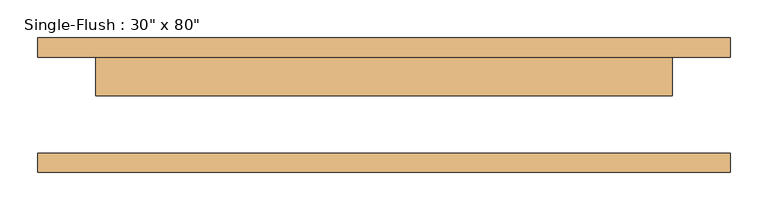
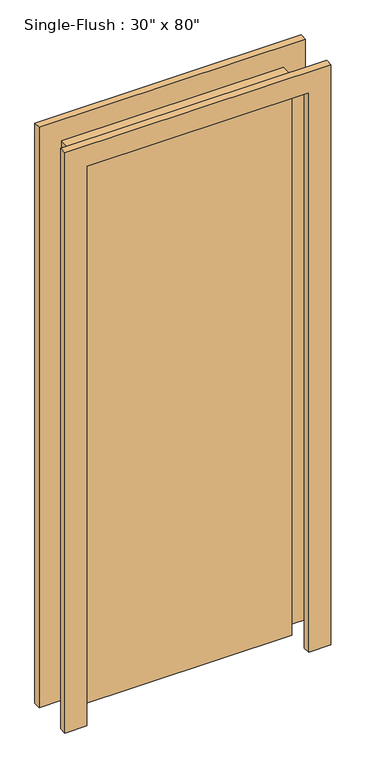
"""IFC4 building model written with IfcOpenShell, lengths in millimetres: door geometry."""

from ifc_helpers import new_model, si_unit, frame, origin, origin_with_axes, place, context, project, spatial, polyline, outline, extrude, source, transform, mapped, element, save


def door_1fe7f57d(model_context):
    return source(origin(), model_context, "Body", "SweptSolid", [
        extrude(outline(polyline([(2108.2, -457.2), (0.0, -457.2), (0.0, -381.0), (2032.0, -381.0), (2032.0, 381.0), (0.0, 381.0), (0.0, 457.2), (2108.2, 457.2), (2108.2, -457.2)])), frame((0.0, 63.5, 0.0), z_axis=(0.0, 1.0, 0.0), x_axis=(0.0, 0.0, 1.0)), (0.0, 0.0, 1.0), 25.4),
        extrude(outline(polyline([(2108.2, 457.2), (2108.2, -457.2), (0.0, -457.2), (0.0, -381.0), (2032.0, -381.0), (2032.0, 381.0), (0.0, 381.0), (0.0, 457.2), (2108.2, 457.2)])), frame((0.0, -88.9, 0.0), z_axis=(0.0, 1.0, 0.0), x_axis=(0.0, 0.0, 1.0)), (0.0, 0.0, 1.0), 25.4),
        extrude(outline(polyline([(381.0, 12.7), (-381.0, 12.7), (-381.0, 63.5), (381.0, 63.5), (381.0, 12.7)])), origin_with_axes(), (0.0, 0.0, 1.0), 2032.0),
    ])


if __name__ == "__main__":
    model = new_model("IFC4")
    model_context = context("Model", 3, world=origin())
    ifc_project = project(units=[si_unit("LENGTHUNIT", "METRE", prefix="MILLI")], contexts=[model_context])
    site = spatial("IfcSite", under=ifc_project)
    building = spatial("IfcBuilding", under=site)
    placement = place(None, origin())
    door_shape = door_1fe7f57d(model_context)
    element("IfcDoor", 1, ObjectType="Single-Flush : 30\" x 80\"", at=placement, inside=building, context=model_context, shape_type="MappedRepresentation", body=[
        mapped(door_shape, transform((0.0, 0.0, 0.0), x_axis=(1.0, 0.0, 0.0), y_axis=(0.0, 1.0, 0.0), z_axis=(0.0, 0.0, 1.0))),
    ])
    save(model, "model.ifc")

# Revit data of these elements
# Type "Single-Flush : 30\" x 80\""
#   Type Mark = "5"
#   Assembly Code = "C1020"
#   Thickness = 0' - 2"
#   Height = 6' - 8"
#   Trim Projection Ext = 0' - 1"
#   Trim Projection Int = 0' - 1"
#   Trim Width = 0' - 3"
#   Width = 2' - 6"
#   Door Material = Door - Panel
#   Frame Material = Door - Frame
#   Function = (empty or 0)
#   Wall Closure = (empty or 0)
# Element 1 (IfcDoor, "Single-Flush : 30\" x 80\"")
#   Materials on its faces: "Door - Frame", "Door - Panel"
# Materials
#   "Door - Panel": class "Wood", colour RGB 114 82 51, transparency 0
#   "Door - Frame": colour RGB 153 76 43, transparency 0
